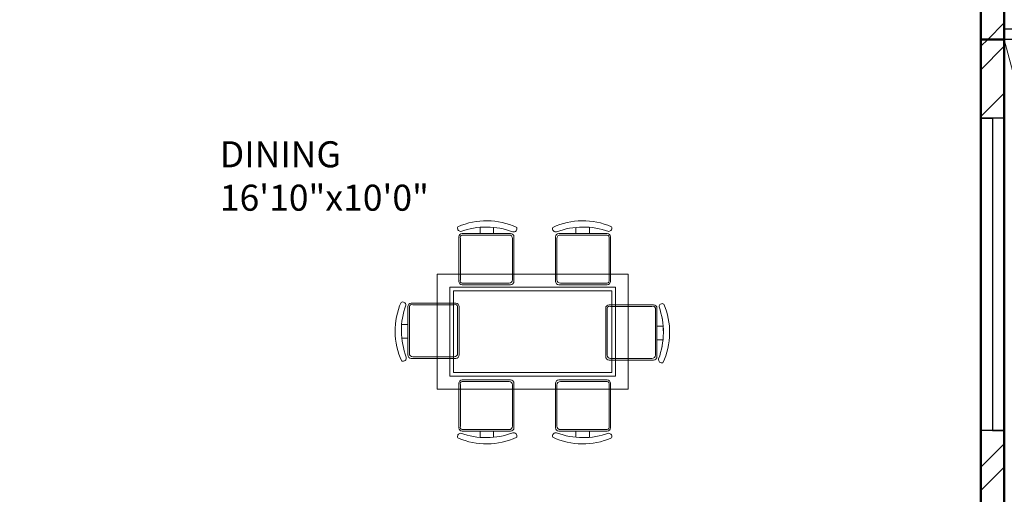
# Model space of a CAD drawing. Units: inches. Extents: x 1901 to 2863, y 888 to 2433.
# Tile 14 of 91: x 2154 to 2343, y 1458 to 1549. Entities that reach past the tile are written whole.
import ezdxf

# ---------------------------------------------------------------- set-up
doc = ezdxf.new("R2010")
doc.units = ezdxf.units.IN
for name, color, linetype, lineweight in [('A-ANNO-SYMB', 8, 'Continuous', 13), ('A-AREA-IDEN', 7, 'Continuous', 18), ('A-FLOR-STRS', 2, 'Continuous', 25), ('A-FURN', 8, 'Continuous', 18), ('A-GLAZ', 3, 'Continuous', 25), ('A-WALL', 7, 'Continuous', 50), ('A-WALL-PATT', 8, 'Continuous', 13)]:
    doc.layers.add(name, color=color, linetype=linetype, lineweight=lineweight)
doc.styles.get("Standard").update_dxf_attribs({"font": 'arial.ttf'})

# ---------------------------------------------------------------- blocks, each defined once
blk = doc.blocks.new('WIN-60')
for p, q in [((0, 4.5), (0, 0)), ((60, 2.25), (60, 4.5)), ((60, 4.5), (60, 0)), ((0, 0), (0, 2.25)), ((0, 2.25), (60, 2.25))]:
    blk.add_line(p, q)

msp = doc.modelspace()

# ---------------------------------------------------------------- hatches: boundary and pattern name
at = {"layer": 'A-WALL-PATT'}
h = msp.add_hatch(dxfattribs=at)
h.set_pattern_fill('ANSI32', color=256)
h.paths.add_polyline_path([(2192.5, 2274.13), (2141.26, 2274.13), (2141.26, 2269.63), (2192.5, 2269.63)])
h.paths.add_polyline_path([(2259.93, 2274.13), (2216.5, 2274.13), (2216.5, 2269.63), (2255.43, 2269.63), (2255.43, 2214.63), (2250.81, 2214.63), (2250.81, 2210.13), (2259.93, 2210.13), (2259.93, 2215.13), (2271.76, 2215.13), (2271.76, 2217.38), (2271.76, 2219.63), (2259.93, 2219.63)])
h.paths.add_polyline_path([(2171.43, 2269.63), (2166.93, 2269.63), (2166.93, 2219.63), (2121.24, 2219.63), (2121.24, 2215.13), (2166.93, 2215.13), (2166.93, 2083.13), (2161.81, 2083.13), (2161.81, 2078.63), (2171.43, 2078.63), (2177, 2078.63), (2177, 2080.88), (2177, 2083.13), (2171.43, 2083.13), (2171.43, 2210.13), (2230.91, 2210.13), (2230.91, 2212.38), (2230.91, 2214.63), (2171.43, 2214.63)])
h.paths.add_polyline_path([(2117.26, 2274.13), (2089.43, 2274.13), (2089.43, 2219.63), (2081.14, 2219.63), (2081.14, 2215.13), (2089.43, 2215.13), (2098, 2215.13), (2098, 2217.38), (2098, 2219.63), (2093.93, 2219.63), (2093.93, 2269.63), (2117.26, 2269.63), (2117.26, 2271.88)])
h.paths.add_polyline_path([(2343.43, 2219.63), (2329.29, 2219.63), (2329.29, 2215.13), (2338.93, 2215.13), (2338.93, 2184.74), (2343.43, 2184.74)])
h.paths.add_polyline_path([(2338.93, 2083.13), (2329.29, 2083.13), (2208.97, 2083.13), (2208.97, 2078.63), (2338.93, 2078.63)])
h.paths.add_polyline_path([(2343.43, 2136.74), (2338.93, 2136.74), (2338.93, 1872.63), (2343.43, 1872.63)])
h.paths.add_polyline_path([(2343.43, 1863.63), (2397.68, 1863.63), (2397.68, 1821.63), (2384.14, 1821.63), (2384.14, 1812.63), (2418.33, 1812.63), (2418.33, 1817.13), (2418.33, 1821.63), (2406.68, 1821.63), (2406.68, 1863.63), (2459.5, 1863.63), (2459.5, 1821.63), (2447.14, 1821.63), (2447.14, 1812.63), (2459.5, 1812.63), (2468.5, 1812.63), (2468.5, 1872.63), (2394.43, 1872.63), (2334.43, 1872.63), (2334.43, 1812.63), (2343.43, 1812.63), (2353.25, 1812.63), (2353.25, 1821.63), (2343.43, 1821.63)])
h.paths.add_polyline_path([(2510.01, 1872.63), (2468.5, 1872.63), (2468.5, 1868.13), (2510.01, 1868.13)])
h.paths.add_polyline_path([(2514.01, 1817.13), (2468.5, 1817.13), (2468.5, 1812.63), (2482.11, 1812.63), (2482.11, 1800.61), (2486.61, 1800.61), (2486.61, 1812.63), (2514.01, 1812.63)])
h.paths.add_polyline_path([(2299.25, 1814.88), (2299.25, 1817.13), (2295.93, 1817.13), (2295.93, 1854.17), (2293.68, 1854.17), (2291.43, 1854.17), (2291.43, 1817.13), (2266.11, 1817.13), (2266.11, 1812.63), (2299.25, 1812.63)])
h.paths.add_polyline_path([(2218.11, 1817.13), (2206.46, 1817.13), (2171.43, 1817.13), (2171.43, 1949.13), (2190.1, 1949.13), (2190.1, 1953.63), (2163.47, 1953.63), (2163.47, 1949.13), (2166.93, 1949.13), (2166.93, 1817.13), (2114.3, 1817.13), (2114.3, 1812.63), (2218.11, 1812.63)])
h.paths.add_polyline_path([(2029.43, 1970.92), (2024.93, 1970.92), (2024.93, 1912.72), (2029.43, 1912.72)])
h.paths.add_polyline_path([(2132.3, 1953.63), (2113.93, 1953.63), (2113.93, 1975.89), (2111.68, 1975.89), (2109.43, 1975.89), (2109.43, 1953.63), (2029.43, 1953.63), (2029.43, 1949.13), (2132.3, 1949.13)])
h.paths.add_polyline_path([(2029.43, 1853.61), (2029.31, 1853.61), (2029.31, 1853.61), (2029.43, 1853.61), (2029.43, 1864.72), (2024.93, 1864.72), (2024.93, 1812.63), (2066.3, 1812.63), (2066.3, 1814.88), (2066.3, 1817.13), (2029.43, 1817.13)])
h.paths.add_polyline_path([(2122.93, 2010.09), (2120.68, 2010.09), (2118.43, 2010.09), (2118.43, 2006.13), (2029.43, 2006.13), (2029.43, 2001.63), (2109.43, 2001.63), (2109.43, 1998.04), (2113.93, 1998.04), (2113.93, 2001.63), (2122.93, 2001.63)])
h.paths.add_polyline_path([(2029.43, 2031.38), (2024.93, 2031.38), (2024.93, 1994.92), (2027.18, 1994.92), (2029.43, 1994.92)])
h.paths.add_polyline_path([(2029.43, 2136.74), (2024.93, 2136.74), (2024.93, 2067.38), (2027.18, 2067.38), (2029.43, 2067.38)])
h.paths.add_polyline_path([(2125.62, 2083.13), (2029.43, 2083.13), (2029.43, 2078.63), (2118.43, 2078.63), (2118.43, 2030.71), (2122.93, 2030.71), (2122.93, 2078.63), (2125.62, 2078.63)])
h.paths.add_polyline_path([(2029.43, 2215.13), (2040.47, 2215.13), (2040.47, 2217.38), (2040.47, 2219.63), (2024.93, 2219.63), (2024.93, 2184.74), (2029.43, 2184.74), (2029.43, 2187.78)])
h.paths.add_polyline_path([(2686.43, 2274.13), (2659.28, 2274.13), (2659.28, 2269.63), (2681.93, 2269.63), (2681.93, 2219.63), (2676.82, 2219.63), (2676.82, 2215.13), (2681.93, 2215.13), (2697.01, 2215.13), (2697.01, 2217.38), (2697.01, 2219.63), (2686.43, 2219.63)])
h.paths.add_polyline_path([(2609.93, 2269.63), (2635.28, 2269.63), (2635.28, 2274.13), (2571.43, 2274.13), (2571.43, 2269.63), (2605.43, 2269.63), (2605.43, 2214.63), (2549.1, 2214.63), (2549.1, 2210.13), (2605.43, 2210.13), (2605.43, 2083.13), (2601.01, 2083.13), (2601.01, 2080.88), (2601.01, 2078.63), (2609.93, 2078.63), (2616.16, 2078.63), (2616.16, 2080.88), (2616.16, 2083.13), (2609.93, 2083.13), (2609.93, 2215.13), (2651.46, 2215.13), (2651.46, 2217.38), (2651.46, 2219.63), (2609.93, 2219.63)])
h.paths.add_polyline_path([(2521.43, 2269.63), (2547.43, 2269.63), (2547.43, 2271.88), (2547.43, 2274.13), (2516.93, 2274.13), (2516.93, 2219.63), (2506.41, 2219.63), (2506.41, 2215.13), (2516.93, 2215.13), (2516.93, 2210.13), (2525.4, 2210.13), (2525.4, 2212.38), (2525.4, 2214.63), (2521.43, 2214.63)])
h.paths.add_polyline_path([(2456.01, 2219.63), (2439.43, 2219.63), (2439.43, 2187.89), (2443.93, 2187.89), (2443.93, 2215.13), (2456.01, 2215.13)])
h.paths.add_polyline_path([(2752.93, 2219.63), (2739.48, 2219.63), (2739.48, 2215.13), (2748.43, 2215.13), (2748.43, 2187.89), (2752.93, 2187.89)])
h.paths.add_polyline_path([(2752.93, 2139.89), (2748.43, 2139.89), (2748.43, 2083.13), (2648.42, 2083.13), (2648.42, 2078.63), (2654.93, 2078.63), (2654.93, 2039.44), (2659.43, 2039.44), (2659.43, 2078.63), (2748.43, 2078.63), (2748.43, 2063.43), (2752.93, 2063.43)])
h.paths.add_polyline_path([(2752.93, 2010.63), (2659.43, 2010.63), (2659.43, 2015.65), (2654.93, 2015.65), (2654.93, 2010.63), (2605.43, 2010.63), (2605.43, 1920.97), (2609.93, 1920.97), (2609.93, 2006.13), (2748.43, 2006.13), (2748.43, 1982.47), (2752.93, 1982.47)])
h.paths.add_polyline_path([(2752.93, 2027.43), (2748.43, 2027.43), (2748.43, 2010.63), (2752.93, 2010.63)])
h.paths.add_polyline_path([(2748.43, 1886.13), (2609.93, 1886.13), (2609.93, 1889.72), (2605.43, 1889.72), (2605.43, 1861.26), (2609.93, 1861.26), (2609.93, 1881.63), (2748.43, 1881.63)])
h.paths.add_polyline_path([(2456.86, 2228.83), (2498.4, 2228.83), (2498.4, 2247.49), (2456.86, 2247.49)], flags=9)
h.paths.add_polyline_path([(2038.6, 2237.42), (2080.17, 2237.42), (2080.17, 2256.08), (2038.6, 2256.08)], flags=9)
h.paths.add_polyline_path([(2292.01, 1062.39), (2539.93, 1062.39), (2539.93, 1099.49), (2292.01, 1099.49)], flags=9)
h.paths.add_polyline_path([(2424.91, 1832.25), (2448.51, 1832.25), (2448.51, 1846.68), (2424.91, 1846.68)], flags=25)
h.paths.add_polyline_path([(2359.08, 1832.25), (2382.68, 1832.25), (2382.68, 1846.68), (2359.08, 1846.68)], flags=25)
h.paths.add_polyline_path([(2352.9, 1684.8), (2367.54, 1684.8), (2367.54, 1697.17), (2352.9, 1697.17)], flags=9)
h.paths.add_polyline_path([(2079.29, 1755.83), (2169.02, 1755.83), (2169.02, 1774.37), (2079.29, 1774.37)], flags=9)
h.paths.add_polyline_path([(2404.09, 1373.86), (2404.09, 1463.59), (2385.54, 1463.59), (2385.54, 1373.86)], flags=9)
h.paths.add_polyline_path([(2268.09, 2236.37), (2309.64, 2236.37), (2309.64, 2255.03), (2268.09, 2255.03)], flags=9)
h.paths.add_polyline_path([(2575.96, 1700.95), (2665.7, 1700.95), (2665.7, 1719.5), (2575.96, 1719.5)], flags=9)
h.paths.add_polyline_path([(2302.96, 1878.47), (2329.52, 1878.47), (2329.52, 1888.78), (2302.96, 1888.78)], flags=9)
h.paths.add_polyline_path([(2097.42, 2240.58), (2126.57, 2240.58), (2126.57, 2259.23), (2097.42, 2259.23)], flags=9)
h.paths.add_polyline_path([(2208.72, 2246.12), (2237.88, 2246.12), (2237.88, 2264.78), (2208.72, 2264.78)], flags=9)
h.paths.add_polyline_path([(2038.15, 1925.96), (2076.99, 1925.96), (2076.99, 1944.62), (2038.15, 1944.62)], flags=9)
h.paths.add_polyline_path([(2239.14, 1926.67), (2288.46, 1926.67), (2288.46, 1945.33), (2239.14, 1945.33)], flags=9)
h.paths.add_polyline_path([(2175.43, 2007.33), (2212.36, 2007.33), (2212.36, 2025.99), (2175.43, 2025.99)], flags=9)
h.paths.add_polyline_path([(2225.03, 2091.79), (2263.87, 2091.79), (2263.87, 2110.45), (2225.03, 2110.45)], flags=9)
h.paths.add_polyline_path([(2035.4, 2098.48), (2074.24, 2098.48), (2074.24, 2117.14), (2035.4, 2117.14)], flags=9)
h.paths.add_polyline_path([(2050.1, 2029.21), (2083.26, 2029.21), (2083.26, 2047.87), (2050.1, 2047.87)], flags=9)
h.paths.add_polyline_path([(2069.68, 1956.72), (2098.83, 1956.72), (2098.83, 1975.38), (2069.68, 1975.38)], flags=25)
h.paths.add_polyline_path([(2328.62, 1753.34), (2361.66, 1753.34), (2361.66, 1771.99), (2328.62, 1771.99)], flags=9)
h.paths.add_polyline_path([(2395.16, 2060.89), (2395.16, 2140.65), (2378.68, 2140.65), (2378.68, 2060.89)], flags=9)
h.paths.add_polyline_path([(2463.73, 2059.02), (2492.89, 2059.02), (2492.89, 2077.68), (2463.73, 2077.68)], flags=9)
h.paths.add_polyline_path([(2458.03, 2181.54), (2496.87, 2181.54), (2496.87, 2200.19), (2458.03, 2200.19)], flags=9)
h.paths.add_polyline_path([(2527.58, 2243.07), (2556.73, 2243.07), (2556.73, 2261.73), (2527.58, 2261.73)], flags=9)
h.paths.add_polyline_path([(2694.46, 2232.77), (2736.03, 2232.77), (2736.03, 2251.42), (2694.46, 2251.42)], flags=9)
h.paths.add_polyline_path([(2637.82, 2249.22), (2666.98, 2249.22), (2666.98, 2267.88), (2637.82, 2267.88)], flags=9)
h.paths.add_polyline_path([(2623.69, 2183.54), (2662.53, 2183.54), (2662.53, 2202.2), (2623.69, 2202.2)], flags=9)
h.paths.add_polyline_path([(2691.97, 2021.5), (2725.12, 2021.5), (2725.12, 2040.16), (2691.97, 2040.16)], flags=9)
h.paths.add_polyline_path([(2621.04, 1975.91), (2662.34, 1975.91), (2662.34, 1994.57), (2621.04, 1994.57)], flags=25)
h.paths.add_polyline_path([(2479.03, 1927.62), (2519.84, 1927.62), (2519.84, 1946.28), (2479.03, 1946.28)], flags=9)
h.paths.add_polyline_path([(2670.94, 1849.08), (2716.01, 1849.08), (2716.01, 1867.73), (2670.94, 1867.73)], flags=9)
h.paths.add_polyline_path([(2523.61, 1782.96), (2550.17, 1782.96), (2550.17, 1793.26), (2523.61, 1793.26)], flags=9)
h.paths.add_polyline_path([(2450.84, 1207.33), (2492.39, 1207.33), (2492.39, 1225.99), (2450.84, 1225.99)], flags=9)
h.paths.add_polyline_path([(2527.75, 1203.84), (2556.91, 1203.84), (2556.91, 1222.5), (2527.75, 1222.5)], flags=9)
h.paths.add_polyline_path([(2639.11, 1207.2), (2668.27, 1207.2), (2668.27, 1225.86), (2639.11, 1225.86)], flags=9)
h.paths.add_polyline_path([(2692.59, 1218.97), (2734.17, 1218.97), (2734.17, 1237.62), (2692.59, 1237.62)], flags=9)
h.paths.add_polyline_path([(2669.27, 1366.33), (2708.11, 1366.33), (2708.11, 1384.99), (2669.27, 1384.99)], flags=9)
h.paths.add_polyline_path([(2463.31, 1358.03), (2502.15, 1358.03), (2502.15, 1376.69), (2463.31, 1376.69)], flags=9)
h.paths.add_polyline_path([(2494.72, 1449.96), (2531.65, 1449.96), (2531.65, 1468.62), (2494.72, 1468.62)], flags=9)
h.paths.add_polyline_path([(2675.57, 1422.16), (2708.72, 1422.16), (2708.72, 1440.81), (2675.57, 1440.81)], flags=9)
h.paths.add_polyline_path([(2685.63, 1493.89), (2714.79, 1493.89), (2714.79, 1512.55), (2685.63, 1512.55)], flags=9)
h.paths.add_polyline_path([(2686.8, 1529.91), (2725.65, 1529.91), (2725.65, 1548.57), (2686.8, 1548.57)], flags=9)
h.paths.add_polyline_path([(2503.65, 1537.99), (2552.97, 1537.99), (2552.97, 1556.65), (2503.65, 1556.65)], flags=9)
h.paths.add_polyline_path([(2291.71, 1643.5), (2318.28, 1643.5), (2318.28, 1653.81), (2291.71, 1653.81)], flags=9)
h.paths.add_polyline_path([(2450.63, 1610.52), (2477.19, 1610.52), (2477.19, 1620.82), (2450.63, 1620.82)], flags=9)
h.paths.add_polyline_path([(2359.99, 1551.81), (2422.25, 1551.81), (2422.25, 1562.12), (2359.99, 1562.12)], flags=9)
h.paths.add_polyline_path([(2280.11, 1249.01), (2321.65, 1249.01), (2321.65, 1267.66), (2280.11, 1267.66)], flags=9)
h.paths.add_polyline_path([(2164.06, 1274.23), (2193.22, 1274.23), (2193.22, 1292.89), (2164.06, 1292.89)], flags=9)
h.paths.add_polyline_path([(2118.21, 1277.69), (2151.25, 1277.69), (2151.25, 1296.35), (2118.21, 1296.35)], flags=9)
h.paths.add_polyline_path([(2031.95, 1268.53), (2073.52, 1268.53), (2073.52, 1287.19), (2031.95, 1287.19)], flags=9)
h.paths.add_polyline_path([(2050.2, 1409.08), (2089.04, 1409.08), (2089.04, 1427.74), (2050.2, 1427.74)], flags=9)
h.paths.add_polyline_path([(2243.74, 1421.03), (2282.58, 1421.03), (2282.58, 1439.69), (2243.74, 1439.69)], flags=9)
h.paths.add_polyline_path([(2190.75, 1509.77), (2231.56, 1509.77), (2231.56, 1528.43), (2190.75, 1528.43)], flags=9)
h.paths.add_polyline_path([(2058.39, 1475.42), (2091.55, 1475.42), (2091.55, 1494.07), (2058.39, 1494.07)], flags=9)
h.paths.add_polyline_path([(2062.45, 1553.09), (2091.6, 1553.09), (2091.6, 1571.75), (2062.45, 1571.75)], flags=9)
h.paths.add_polyline_path([(2219.52, 1590.37), (2266.15, 1590.37), (2266.15, 1609.02), (2219.52, 1609.02)], flags=9)
h.paths.add_polyline_path([(2041.07, 1584.19), (2079.91, 1584.19), (2079.91, 1602.85), (2041.07, 1602.85)], flags=9)
h = msp.add_hatch(dxfattribs=at)
h.set_pattern_fill('ANSI32', color=256)
h.paths.add_polyline_path([(2443.93, 2139.89), (2439.43, 2139.89), (2439.43, 2069.35), (2441.68, 2069.35), (2443.93, 2069.35), (2443.93, 2078.63), (2521.93, 2078.63), (2521.93, 2075.07), (2524.18, 2075.07), (2526.43, 2075.07), (2526.43, 2078.63), (2571.75, 2078.63), (2571.75, 2080.88), (2571.75, 2083.13), (2443.93, 2083.13)])
h.paths.add_polyline_path([(2526.43, 2054.63), (2524.18, 2054.63), (2521.93, 2054.63), (2521.93, 2030.63), (2443.93, 2030.63), (2443.93, 2045.35), (2439.43, 2045.35), (2439.43, 1983.87), (2443.93, 1983.87), (2443.93, 2026.13), (2521.93, 2026.13), (2526.43, 2026.13)])
h.paths.add_polyline_path([(2443.93, 1923.87), (2439.43, 1923.87), (2439.43, 1872.63), (2443.93, 1872.63)])
h.paths.add_polyline_path([(2636.23, 1766.13), (2609.93, 1766.13), (2609.93, 1779.79), (2605.43, 1779.79), (2605.43, 1766.13), (2486.61, 1766.13), (2486.61, 1770.67), (2482.11, 1770.67), (2482.11, 1766.13), (2482.11, 1761.63), (2636.23, 1761.63), (2636.23, 1763.88)])
h.paths.add_polyline_path([(2519.54, 1663.38), (2519.54, 1665.63), (2494.93, 1665.63), (2481.83, 1665.63), (2481.83, 1663.38), (2481.83, 1661.13), (2490.43, 1661.13), (2490.43, 1640.16), (2494.93, 1640.16), (2494.93, 1661.13), (2519.54, 1661.13)])
h.paths.add_polyline_path([(2443.93, 1712.13), (2443.93, 1716.63), (2414.46, 1716.63), (2414.46, 1712.13), (2439.43, 1712.13), (2439.43, 1545.51), (2443.93, 1545.51), (2443.93, 1661.13), (2448.47, 1661.13), (2448.47, 1665.63), (2443.93, 1665.63)])
h.paths.add_polyline_path([(2343.43, 1712.13), (2365.52, 1712.13), (2365.52, 1714.38), (2365.52, 1716.63), (2333.87, 1716.63), (2333.87, 1714.38), (2333.87, 1712.13), (2338.93, 1712.13), (2338.93, 1575.63), (2338.93, 1545.51), (2343.43, 1545.51), (2343.43, 1547.51), (2343.43, 1580.13)])
h.paths.add_polyline_path([(2752.93, 1665.63), (2579.54, 1665.63), (2579.54, 1661.13), (2615.93, 1661.13), (2615.93, 1529.13), (2598.93, 1529.13), (2598.93, 1524.63), (2623.13, 1524.63), (2623.13, 1526.88), (2623.13, 1529.13), (2620.43, 1529.13), (2620.43, 1661.13), (2748.43, 1661.13), (2748.43, 1633.5), (2752.93, 1633.5)])
h.paths.add_polyline_path([(2752.93, 1419.93), (2748.43, 1419.93), (2748.43, 1400.13), (2659.43, 1400.13), (2659.43, 1444.33), (2657.18, 1444.33), (2654.93, 1444.33), (2654.93, 1400.13), (2643.65, 1400.13), (2643.65, 1395.63), (2748.43, 1395.63), (2748.43, 1364.04), (2752.93, 1364.04)])
h.paths.add_polyline_path([(2752.93, 1492.88), (2748.43, 1492.88), (2748.43, 1476.63), (2667.43, 1476.63), (2667.43, 1479.71), (2665.18, 1479.71), (2662.93, 1479.71), (2662.93, 1476.63), (2654.93, 1476.63), (2654.93, 1469.54), (2659.43, 1469.54), (2659.43, 1472.13), (2748.43, 1472.13), (2748.43, 1455.93), (2752.93, 1455.93)])
h.paths.add_polyline_path([(2752.93, 1304.04), (2748.43, 1304.04), (2748.43, 1263.63), (2738.66, 1263.63), (2738.66, 1259.13), (2752.93, 1259.13)])
h.paths.add_polyline_path([(2685.93, 1259.13), (2695.49, 1259.13), (2695.49, 1261.38), (2695.49, 1263.63), (2677.84, 1263.63), (2677.84, 1261.38), (2677.84, 1259.13), (2681.43, 1259.13), (2681.43, 1203.63), (2653.28, 1203.63), (2653.28, 1199.13), (2685.93, 1199.13), (2685.93, 1203.63)])
h.paths.add_polyline_path([(2609.43, 1395.63), (2611.85, 1395.63), (2611.85, 1400.13), (2598.89, 1400.13), (2598.89, 1397.88), (2598.89, 1395.63), (2604.93, 1395.63), (2604.93, 1268.13), (2554.73, 1268.13), (2554.73, 1265.88), (2554.73, 1263.63), (2604.93, 1263.63), (2604.93, 1203.63), (2571.31, 1203.63), (2571.31, 1199.13), (2604.93, 1199.13), (2629.28, 1199.13), (2629.28, 1201.38), (2629.28, 1203.63), (2609.43, 1203.63), (2609.43, 1258.63), (2609.43, 1259.13), (2654.8, 1259.13), (2654.8, 1263.63), (2609.43, 1263.63)])
h.paths.add_polyline_path([(2443.93, 1304.04), (2439.43, 1304.04), (2439.43, 1259.13), (2443.93, 1259.13), (2456.16, 1259.13), (2456.16, 1261.38), (2456.16, 1263.63), (2443.93, 1263.63)])
h.paths.add_polyline_path([(2525.43, 1263.63), (2531.78, 1263.63), (2531.78, 1268.13), (2520.93, 1268.13), (2520.93, 1263.63), (2511.41, 1263.63), (2511.41, 1259.13), (2520.93, 1259.13), (2520.93, 1199.13), (2547.31, 1199.13), (2547.31, 1201.38), (2547.31, 1203.63), (2525.43, 1203.63)])
h.paths.add_polyline_path([(2443.93, 1434.84), (2439.43, 1434.84), (2439.43, 1364.04), (2441.68, 1364.04), (2443.93, 1364.04)])
h.paths.add_polyline_path([(2567.13, 1400.13), (2443.93, 1400.13), (2443.93, 1395.63), (2567.13, 1395.63)])
h.paths.add_polyline_path([(2443.93, 1545.51), (2439.43, 1545.51), (2439.43, 1494.84), (2443.93, 1494.84)])
h.paths.add_polyline_path([(2494.93, 1553.35), (2492.68, 1553.35), (2490.43, 1553.35), (2490.43, 1524.63), (2494.93, 1524.63), (2525.94, 1524.63), (2525.94, 1526.88), (2525.94, 1529.13), (2494.93, 1529.13)])
h.paths.add_polyline_path([(2752.93, 1573.5), (2748.43, 1573.5), (2748.43, 1529.13), (2657.76, 1529.13), (2657.76, 1524.63), (2662.93, 1524.63), (2662.93, 1498.63), (2667.43, 1498.63), (2667.43, 1524.63), (2748.43, 1524.63), (2748.43, 1516.88), (2752.93, 1516.88)])
h.paths.add_polyline_path([(2038.6, 2237.42), (2080.17, 2237.42), (2080.17, 2256.08), (2038.6, 2256.08)], flags=9)
h.paths.add_polyline_path([(2292.01, 1062.39), (2539.93, 1062.39), (2539.93, 1099.49), (2292.01, 1099.49)], flags=9)
h.paths.add_polyline_path([(2424.91, 1832.25), (2448.51, 1832.25), (2448.51, 1846.68), (2424.91, 1846.68)], flags=9)
h.paths.add_polyline_path([(2359.08, 1832.25), (2382.68, 1832.25), (2382.68, 1846.68), (2359.08, 1846.68)], flags=9)
h.paths.add_polyline_path([(2352.9, 1684.8), (2367.54, 1684.8), (2367.54, 1697.17), (2352.9, 1697.17)], flags=9)
h.paths.add_polyline_path([(2079.29, 1755.83), (2169.02, 1755.83), (2169.02, 1774.37), (2079.29, 1774.37)], flags=9)
h.paths.add_polyline_path([(2404.09, 1373.86), (2404.09, 1463.59), (2385.54, 1463.59), (2385.54, 1373.86)], flags=9)
h.paths.add_polyline_path([(2268.09, 2236.37), (2309.64, 2236.37), (2309.64, 2255.03), (2268.09, 2255.03)], flags=9)
h.paths.add_polyline_path([(2575.96, 1700.95), (2665.7, 1700.95), (2665.7, 1719.5), (2575.96, 1719.5)], flags=9)
h.paths.add_polyline_path([(2302.96, 1878.47), (2329.52, 1878.47), (2329.52, 1888.78), (2302.96, 1888.78)], flags=9)
h.paths.add_polyline_path([(2097.42, 2240.58), (2126.57, 2240.58), (2126.57, 2259.23), (2097.42, 2259.23)], flags=9)
h.paths.add_polyline_path([(2208.72, 2246.12), (2237.88, 2246.12), (2237.88, 2264.78), (2208.72, 2264.78)], flags=9)
h.paths.add_polyline_path([(2038.15, 1925.96), (2076.99, 1925.96), (2076.99, 1944.62), (2038.15, 1944.62)], flags=9)
h.paths.add_polyline_path([(2239.14, 1926.67), (2288.46, 1926.67), (2288.46, 1945.33), (2239.14, 1945.33)], flags=9)
h.paths.add_polyline_path([(2175.43, 2007.33), (2212.36, 2007.33), (2212.36, 2025.99), (2175.43, 2025.99)], flags=9)
h.paths.add_polyline_path([(2225.03, 2091.79), (2263.87, 2091.79), (2263.87, 2110.45), (2225.03, 2110.45)], flags=9)
h.paths.add_polyline_path([(2035.4, 2098.48), (2074.24, 2098.48), (2074.24, 2117.14), (2035.4, 2117.14)], flags=9)
h.paths.add_polyline_path([(2050.1, 2029.21), (2083.26, 2029.21), (2083.26, 2047.87), (2050.1, 2047.87)], flags=9)
h.paths.add_polyline_path([(2069.68, 1956.72), (2098.83, 1956.72), (2098.83, 1975.38), (2069.68, 1975.38)], flags=9)
h.paths.add_polyline_path([(2328.62, 1753.34), (2361.66, 1753.34), (2361.66, 1771.99), (2328.62, 1771.99)], flags=9)
h.paths.add_polyline_path([(2395.16, 2060.89), (2395.16, 2140.65), (2378.68, 2140.65), (2378.68, 2060.89)], flags=9)
h.paths.add_polyline_path([(2463.73, 2059.02), (2492.89, 2059.02), (2492.89, 2077.68), (2463.73, 2077.68)], flags=9)
h.paths.add_polyline_path([(2458.03, 2181.54), (2496.87, 2181.54), (2496.87, 2200.19), (2458.03, 2200.19)], flags=9)
h.paths.add_polyline_path([(2456.86, 2228.83), (2498.4, 2228.83), (2498.4, 2247.49), (2456.86, 2247.49)], flags=9)
h.paths.add_polyline_path([(2527.58, 2243.07), (2556.73, 2243.07), (2556.73, 2261.73), (2527.58, 2261.73)], flags=9)
h.paths.add_polyline_path([(2694.46, 2232.77), (2736.03, 2232.77), (2736.03, 2251.42), (2694.46, 2251.42)], flags=9)
h.paths.add_polyline_path([(2637.82, 2249.22), (2666.98, 2249.22), (2666.98, 2267.88), (2637.82, 2267.88)], flags=9)
h.paths.add_polyline_path([(2623.69, 2183.54), (2662.53, 2183.54), (2662.53, 2202.2), (2623.69, 2202.2)], flags=9)
h.paths.add_polyline_path([(2691.97, 2021.5), (2725.12, 2021.5), (2725.12, 2040.16), (2691.97, 2040.16)], flags=9)
h.paths.add_polyline_path([(2621.04, 1975.91), (2662.34, 1975.91), (2662.34, 1994.57), (2621.04, 1994.57)], flags=9)
h.paths.add_polyline_path([(2479.03, 1927.62), (2519.84, 1927.62), (2519.84, 1946.28), (2479.03, 1946.28)], flags=9)
h.paths.add_polyline_path([(2670.94, 1849.08), (2716.01, 1849.08), (2716.01, 1867.73), (2670.94, 1867.73)], flags=9)
h.paths.add_polyline_path([(2523.61, 1782.96), (2550.17, 1782.96), (2550.17, 1793.26), (2523.61, 1793.26)], flags=9)
h.paths.add_polyline_path([(2450.84, 1207.33), (2492.39, 1207.33), (2492.39, 1225.99), (2450.84, 1225.99)], flags=9)
h.paths.add_polyline_path([(2527.75, 1203.84), (2556.91, 1203.84), (2556.91, 1222.5), (2527.75, 1222.5)], flags=9)
h.paths.add_polyline_path([(2639.11, 1207.2), (2668.27, 1207.2), (2668.27, 1225.86), (2639.11, 1225.86)], flags=9)
h.paths.add_polyline_path([(2692.59, 1218.97), (2734.17, 1218.97), (2734.17, 1237.62), (2692.59, 1237.62)], flags=9)
h.paths.add_polyline_path([(2669.27, 1366.33), (2708.11, 1366.33), (2708.11, 1384.99), (2669.27, 1384.99)], flags=25)
h.paths.add_polyline_path([(2463.31, 1358.03), (2502.15, 1358.03), (2502.15, 1376.69), (2463.31, 1376.69)], flags=9)
h.paths.add_polyline_path([(2494.72, 1449.96), (2531.65, 1449.96), (2531.65, 1468.62), (2494.72, 1468.62)], flags=9)
h.paths.add_polyline_path([(2675.57, 1422.16), (2708.72, 1422.16), (2708.72, 1440.81), (2675.57, 1440.81)], flags=25)
h.paths.add_polyline_path([(2685.63, 1493.89), (2714.79, 1493.89), (2714.79, 1512.55), (2685.63, 1512.55)], flags=9)
h.paths.add_polyline_path([(2686.8, 1529.91), (2725.65, 1529.91), (2725.65, 1548.57), (2686.8, 1548.57)], flags=25)
h.paths.add_polyline_path([(2503.65, 1537.99), (2552.97, 1537.99), (2552.97, 1556.65), (2503.65, 1556.65)], flags=9)
h.paths.add_polyline_path([(2291.71, 1643.5), (2318.28, 1643.5), (2318.28, 1653.81), (2291.71, 1653.81)], flags=9)
h.paths.add_polyline_path([(2450.63, 1610.52), (2477.19, 1610.52), (2477.19, 1620.82), (2450.63, 1620.82)], flags=9)
h.paths.add_polyline_path([(2359.99, 1551.81), (2422.25, 1551.81), (2422.25, 1562.12), (2359.99, 1562.12)], flags=9)
h.paths.add_polyline_path([(2280.11, 1249.01), (2321.65, 1249.01), (2321.65, 1267.66), (2280.11, 1267.66)], flags=9)
h.paths.add_polyline_path([(2164.06, 1274.23), (2193.22, 1274.23), (2193.22, 1292.89), (2164.06, 1292.89)], flags=9)
h.paths.add_polyline_path([(2118.21, 1277.69), (2151.25, 1277.69), (2151.25, 1296.35), (2118.21, 1296.35)], flags=9)
h.paths.add_polyline_path([(2031.95, 1268.53), (2073.52, 1268.53), (2073.52, 1287.19), (2031.95, 1287.19)], flags=9)
h.paths.add_polyline_path([(2050.2, 1409.08), (2089.04, 1409.08), (2089.04, 1427.74), (2050.2, 1427.74)], flags=9)
h.paths.add_polyline_path([(2243.74, 1421.03), (2282.58, 1421.03), (2282.58, 1439.69), (2243.74, 1439.69)], flags=9)
h.paths.add_polyline_path([(2190.75, 1509.77), (2231.56, 1509.77), (2231.56, 1528.43), (2190.75, 1528.43)], flags=9)
h.paths.add_polyline_path([(2058.39, 1475.42), (2091.55, 1475.42), (2091.55, 1494.07), (2058.39, 1494.07)], flags=9)
h.paths.add_polyline_path([(2062.45, 1553.09), (2091.6, 1553.09), (2091.6, 1571.75), (2062.45, 1571.75)], flags=9)
h.paths.add_polyline_path([(2219.52, 1590.37), (2266.15, 1590.37), (2266.15, 1609.02), (2219.52, 1609.02)], flags=9)
h.paths.add_polyline_path([(2041.07, 1584.19), (2079.91, 1584.19), (2079.91, 1602.85), (2041.07, 1602.85)], flags=9)
h = msp.add_hatch(dxfattribs=at)
h.set_pattern_fill('ANSI32', color=256)
h.paths.add_polyline_path([(2182.93, 1716.63), (2024.93, 1716.63), (2024.93, 1681.7), (2029.33, 1681.7), (2029.33, 1712.13), (2154.33, 1712.13), (2154.33, 1580.13), (2148.52, 1580.13), (2148.52, 1577.88), (2148.52, 1575.63), (2194.93, 1575.63), (2194.93, 1580.13), (2158.83, 1580.13), (2158.83, 1712.13), (2182.93, 1712.13)])
h.paths.add_polyline_path([(2301.07, 1716.63), (2242.93, 1716.63), (2242.93, 1712.13), (2283.83, 1712.13), (2283.83, 1685.54), (2288.33, 1685.54), (2288.33, 1712.13), (2301.07, 1712.13)])
h.paths.add_polyline_path([(2288.33, 1600.41), (2286.08, 1600.41), (2283.83, 1600.41), (2283.83, 1580.13), (2270.6, 1580.13), (2270.6, 1575.63), (2288.33, 1575.63)])
h.paths.add_polyline_path([(2295.93, 1953.63), (2271.45, 1953.63), (2271.45, 1949.13), (2291.43, 1949.13), (2291.43, 1941.24), (2295.93, 1941.24)])
h.paths.add_polyline_path([(2098.38, 1244.13), (2082.33, 1244.13), (2082.33, 1302.13), (2086.52, 1302.13), (2086.52, 1306.63), (2067.46, 1306.63), (2067.46, 1302.13), (2077.83, 1302.13), (2077.83, 1239.63), (2098.38, 1239.63), (2098.38, 1241.88)])
h.paths.add_polyline_path([(2217.31, 1306.63), (2158.83, 1306.63), (2158.83, 1451.63), (2162.72, 1451.63), (2162.72, 1453.88), (2162.72, 1456.13), (2154.33, 1456.13), (2154.33, 1443.13), (2151.91, 1443.13), (2151.91, 1438.63), (2154.33, 1438.63), (2154.33, 1306.63), (2109.31, 1306.63), (2109.31, 1304.38), (2109.31, 1302.13), (2154.33, 1302.13), (2154.33, 1244.13), (2122.38, 1244.13), (2122.38, 1239.63), (2154.33, 1239.63), (2154.33, 1223.63), (2163.33, 1223.63), (2181.01, 1223.63), (2181.01, 1225.88), (2181.01, 1228.13), (2163.33, 1228.13), (2163.33, 1258.22), (2158.83, 1258.22), (2158.83, 1302.13), (2217.31, 1302.13)])
h.paths.add_polyline_path([(2259.99, 1306.63), (2238.3, 1306.63), (2238.3, 1304.38), (2238.3, 1302.13), (2242.83, 1302.13), (2242.83, 1228.13), (2205.01, 1228.13), (2205.01, 1223.63), (2247.33, 1223.63), (2247.33, 1302.13), (2259.99, 1302.13), (2259.99, 1304.38)])
h.paths.add_polyline_path([(2343.43, 1361.7), (2338.93, 1361.7), (2338.93, 1306.63), (2322.38, 1306.63), (2322.38, 1302.13), (2343.43, 1302.13)])
h.paths.add_polyline_path([(2343.43, 1470.4), (2338.93, 1470.4), (2338.93, 1456.13), (2193.73, 1456.13), (2193.73, 1453.88), (2193.73, 1451.63), (2338.93, 1451.63), (2338.93, 1421.7), (2343.43, 1421.7)])
h.paths.add_polyline_path([(2343.43, 1545.51), (2338.93, 1545.51), (2338.93, 1530.4), (2343.43, 1530.4)])
h.paths.add_polyline_path([(2029.33, 1466.83), (2024.93, 1466.83), (2024.93, 1409.82), (2029.33, 1409.82)])
h.paths.add_polyline_path([(2122.84, 1440.88), (2122.84, 1443.13), (2121.83, 1443.13), (2121.83, 1498.18), (2119.58, 1498.18), (2117.33, 1498.18), (2117.33, 1443.13), (2029.33, 1443.13), (2029.33, 1438.63), (2122.84, 1438.63)])
h.paths.add_polyline_path([(2029.33, 1543.05), (2024.93, 1543.05), (2024.93, 1502.83), (2029.33, 1502.83)])
h.paths.add_polyline_path([(2029.33, 1621.7), (2024.93, 1621.7), (2024.93, 1567.05), (2027.13, 1567.05), (2029.33, 1567.05), (2029.33, 1575.63), (2109.33, 1575.63), (2109.33, 1554.71), (2113.83, 1554.71), (2113.83, 1575.63), (2115.8, 1575.63), (2115.8, 1577.88), (2115.8, 1580.13), (2029.33, 1580.13)])
h.paths.add_polyline_path([(2121.83, 1527.63), (2117.33, 1527.63), (2113.83, 1527.63), (2113.83, 1533.01), (2111.58, 1533.01), (2109.33, 1533.01), (2109.33, 1527.63), (2029.33, 1527.63), (2029.33, 1523.13), (2117.33, 1523.13), (2117.33, 1519.43), (2121.83, 1519.43)])
h.paths.add_polyline_path([(2029.33, 1349.82), (2024.93, 1349.82), (2024.93, 1302.13), (2036.28, 1302.13), (2036.28, 1306.63), (2029.33, 1306.63)])

# ---------------------------------------------------------------- linework, layer by layer
at = {"layer": 'A-ANNO-SYMB'}
msp.add_line((2343.43, 1545.51), (2439.43, 1181.13), dxfattribs=at)
at = {"layer": 'A-FLOR-STRS'}
for p, q in [((2343.43, 1545.51), (2343.43, 1547.51)), ((2343.43, 1547.51), (2439.43, 1547.51)), ((2439.43, 1545.51), (2343.43, 1545.51))]:
    msp.add_line(p, q, dxfattribs=at)
at = {"layer": 'A-FURN'}
for points in [[(2239.02, 1508.63, -0.175809), (2249.03, 1508.55, 0.578392), (2249.78, 1509.39, 0.214524), (2238.49, 1509.54, 0.552014), (2239.02, 1508.63, -0.065079)], [(2239.02, 1508.63, -0.175809), (2249.03, 1508.55, 0.578392), (2249.78, 1509.39, 0.214524), (2238.49, 1509.54, 0.552014), (2239.02, 1508.63, -0.065079)], [(2245.34, 1508.23), (2245.34, 1509.4, -0.064759)], [(2245.34, 1508.23), (2245.34, 1509.4, -0.064759)], [(2257.45, 1508.55, -0.578392), (2256.69, 1509.39, -0.214524), (2267.98, 1509.54, -0.552014), (2267.45, 1508.63, 0.175809), (2257.45, 1508.55)], [(2257.45, 1508.55, -0.578392), (2256.69, 1509.39, -0.214524), (2267.98, 1509.54, -0.552014), (2267.45, 1508.63, 0.175809), (2257.45, 1508.55)], [(2261.13, 1508.23), (2261.13, 1509.4, 0.064759)], [(2261.13, 1508.23), (2261.13, 1509.4, 0.064759)], [(2248.6, 1508.23), (2239.31, 1508.23, 0.414214), (2238.66, 1507.58), (2238.66, 1499.04, 0.414214), (2239.31, 1498.39), (2248.6, 1498.39, 0.414214), (2249.25, 1499.04), (2249.25, 1507.58, 0.414214), (2248.6, 1508.23)], [(2248.6, 1508.23), (2239.31, 1508.23, 0.414214), (2238.66, 1507.58), (2238.66, 1499.04, 0.414214), (2239.31, 1498.39), (2248.6, 1498.39, 0.414214), (2249.25, 1499.04), (2249.25, 1507.58, 0.414214), (2248.6, 1508.23)], [(2267.16, 1508.23, -0.414214), (2267.81, 1507.58), (2267.81, 1499.04, -0.414214), (2267.16, 1498.39), (2257.87, 1498.39, -0.414214), (2257.22, 1499.04), (2257.22, 1507.58, -0.414214), (2257.87, 1508.23), (2267.16, 1508.23)], [(2267.16, 1508.23, -0.414214), (2267.81, 1507.58), (2267.81, 1499.04, -0.414214), (2267.16, 1498.39), (2257.87, 1498.39, -0.414214), (2257.22, 1499.04), (2257.22, 1507.58, -0.414214), (2257.87, 1508.23), (2267.16, 1508.23)], [(2228.56, 1484.47, -0.578392), (2227.72, 1483.72, -0.214524), (2227.57, 1495.01, -0.552014), (2228.48, 1494.48, 0.175809), (2228.56, 1484.47)], [(2228.56, 1484.47, -0.578392), (2227.72, 1483.72, -0.214524), (2227.57, 1495.01, -0.552014), (2228.48, 1494.48, 0.175809), (2228.56, 1484.47)], [(2228.88, 1494.18, -0.414214), (2229.53, 1494.83), (2238.07, 1494.83, -0.414214), (2238.72, 1494.18), (2238.72, 1484.9, -0.414214), (2238.07, 1484.25), (2229.53, 1484.25, -0.414214), (2228.88, 1484.9), (2228.88, 1494.18)], [(2228.88, 1494.18, -0.414214), (2229.53, 1494.83), (2238.07, 1494.83, -0.414214), (2238.72, 1494.18), (2238.72, 1484.9, -0.414214), (2238.07, 1484.25), (2229.53, 1484.25, -0.414214), (2228.88, 1484.9), (2228.88, 1494.18)], [(2276.71, 1493.87, 0.414214), (2276.06, 1494.52), (2267.52, 1494.52, 0.414214), (2266.87, 1493.87), (2266.87, 1484.58, 0.414214), (2267.52, 1483.93), (2276.06, 1483.93, 0.414214), (2276.71, 1484.58), (2276.71, 1493.87)], [(2276.71, 1493.87, 0.414214), (2276.06, 1494.52), (2267.52, 1494.52, 0.414214), (2266.87, 1493.87), (2266.87, 1484.58, 0.414214), (2267.52, 1483.93), (2276.06, 1483.93, 0.414214), (2276.71, 1484.58), (2276.71, 1493.87)], [(2277.11, 1494.16, -0.175809), (2277.03, 1484.16, 0.578392), (2277.86, 1483.4, 0.214524), (2278.02, 1494.69, 0.552014), (2277.11, 1494.16, -0.065079)], [(2277.11, 1494.16, -0.175809), (2277.03, 1484.15, 0.578392), (2277.86, 1483.4, 0.214524), (2278.02, 1494.69, 0.552014), (2277.11, 1494.16, -0.065079)], [(2228.88, 1488.16), (2227.71, 1488.16, 0.064759)], [(2228.88, 1488.16), (2227.71, 1488.16, 0.064759)], [(2276.71, 1487.84), (2277.88, 1487.84, -0.064759)], [(2276.71, 1487.84), (2277.88, 1487.84, -0.064759)], [(2248.6, 1470.27), (2239.31, 1470.27, -0.414214), (2238.66, 1470.92), (2238.66, 1479.46, -0.414214), (2239.31, 1480.11), (2248.6, 1480.11, -0.414214), (2249.25, 1479.46), (2249.25, 1470.92, -0.414214), (2248.6, 1470.27)], [(2248.6, 1470.27), (2239.31, 1470.27, -0.414214), (2238.66, 1470.92), (2238.66, 1479.46, -0.414214), (2239.31, 1480.11), (2248.6, 1480.11, -0.414214), (2249.25, 1479.46), (2249.25, 1470.92, -0.414214), (2248.6, 1470.27)], [(2267.16, 1470.27, 0.414214), (2267.81, 1470.92), (2267.81, 1479.46, 0.414214), (2267.16, 1480.11), (2257.87, 1480.11, 0.414214), (2257.22, 1479.46), (2257.22, 1470.92, 0.414214), (2257.87, 1470.27), (2267.16, 1470.27)], [(2267.16, 1470.27, 0.414214), (2267.81, 1470.92), (2267.81, 1479.46, 0.414214), (2267.16, 1480.11), (2257.87, 1480.11, 0.414214), (2257.22, 1479.46), (2257.22, 1470.92, 0.414214), (2257.87, 1470.27), (2267.16, 1470.27)], [(2249.03, 1469.94, -0.578392), (2249.78, 1469.11, -0.214524), (2238.49, 1468.96, -0.552014), (2239.02, 1469.87, 0.175809), (2249.03, 1469.94)], [(2249.03, 1469.94, -0.578392), (2249.78, 1469.11, -0.214524), (2238.49, 1468.96, -0.552014), (2239.02, 1469.87, 0.175809), (2249.03, 1469.94)], [(2245.34, 1470.27), (2245.34, 1469.1, 0.064759)], [(2245.34, 1470.27), (2245.34, 1469.1, 0.064759)], [(2267.45, 1469.87, -0.175809), (2257.45, 1469.94, 0.578392), (2256.69, 1469.11, 0.214524), (2267.98, 1468.96, 0.552014), (2267.45, 1469.87, -0.065079)], [(2267.45, 1469.87, -0.175809), (2257.45, 1469.94, 0.578392), (2256.69, 1469.11, 0.214524), (2267.98, 1468.96, 0.552014), (2267.45, 1469.87, -0.065079)], [(2261.13, 1470.27), (2261.13, 1469.1, -0.064759)], [(2261.13, 1470.27), (2261.13, 1469.1, -0.064759)]]:
    msp.add_lwpolyline(points, format="xyb", dxfattribs=at)
for points in [[(2242.74, 1509.42), (2242.74, 1508.23)], [(2242.74, 1509.42), (2242.74, 1508.23)], [(2263.73, 1509.42), (2263.73, 1508.23)], [(2263.73, 1509.42), (2263.73, 1508.23)], [(2227.69, 1490.76), (2228.88, 1490.76)], [(2227.69, 1490.76), (2228.88, 1490.76)], [(2277.9, 1490.44), (2276.71, 1490.44)], [(2277.9, 1490.44), (2276.71, 1490.44)], [(2242.74, 1469.07), (2242.74, 1470.27)], [(2242.74, 1469.07), (2242.74, 1470.27)], [(2263.73, 1469.07), (2263.73, 1470.27)], [(2263.73, 1469.07), (2263.73, 1470.27)]]:
    msp.add_lwpolyline(points, dxfattribs=at)
for points in [[(2239.32, 1507.94), (2248.31, 1507.94, -0.414214), (2248.96, 1507.29), (2248.96, 1499.33, -0.414214), (2248.31, 1498.68), (2239.32, 1498.68, -0.512069), (2238.96, 1499.33), (2238.96, 1507.29, -0.512069)], [(2239.32, 1507.94), (2248.31, 1507.94, -0.414214), (2248.96, 1507.29), (2248.96, 1499.33, -0.414214), (2248.31, 1498.68), (2239.32, 1498.68, -0.512069), (2238.96, 1499.33), (2238.96, 1507.29, -0.512069)], [(2267.15, 1507.94), (2258.16, 1507.94, 0.414214), (2257.51, 1507.29), (2257.51, 1499.33, 0.414214), (2258.16, 1498.68), (2267.15, 1498.68, 0.512069), (2267.52, 1499.33), (2267.52, 1507.29, 0.512069)], [(2267.15, 1507.94), (2258.16, 1507.94, 0.414214), (2257.51, 1507.29), (2257.51, 1499.33, 0.414214), (2258.16, 1498.68), (2267.15, 1498.68, 0.512069), (2267.52, 1499.33), (2267.52, 1507.29, 0.512069)], [(2229.17, 1494.18), (2229.17, 1485.19, 0.414214), (2229.82, 1484.54), (2237.78, 1484.54, 0.414214), (2238.43, 1485.19), (2238.43, 1494.18, 0.512069), (2237.78, 1494.54), (2229.82, 1494.54, 0.512069)], [(2229.17, 1494.18), (2229.17, 1485.19, 0.414214), (2229.82, 1484.54), (2237.78, 1484.54, 0.414214), (2238.43, 1485.19), (2238.43, 1494.18, 0.512069), (2237.78, 1494.54), (2229.82, 1494.54, 0.512069)], [(2276.41, 1493.86), (2276.41, 1484.87, -0.414214), (2275.76, 1484.22), (2267.81, 1484.22, -0.414214), (2267.16, 1484.87), (2267.16, 1493.86, -0.512069), (2267.81, 1494.22), (2275.76, 1494.22, -0.512069)], [(2276.41, 1493.86), (2276.41, 1484.87, -0.414214), (2275.76, 1484.22), (2267.81, 1484.22, -0.414214), (2267.16, 1484.87), (2267.16, 1493.86, -0.512069), (2267.81, 1494.22), (2275.76, 1494.22, -0.512069)], [(2239.32, 1470.56), (2248.31, 1470.56, 0.414214), (2248.96, 1471.21), (2248.96, 1479.17, 0.414214), (2248.31, 1479.82), (2239.32, 1479.82, 0.512069), (2238.96, 1479.17), (2238.96, 1471.21, 0.512069)], [(2239.32, 1470.56), (2248.31, 1470.56, 0.414214), (2248.96, 1471.21), (2248.96, 1479.17, 0.414214), (2248.31, 1479.82), (2239.32, 1479.82, 0.512069), (2238.96, 1479.17), (2238.96, 1471.21, 0.512069)], [(2267.15, 1470.56), (2258.16, 1470.56, -0.414214), (2257.51, 1471.21), (2257.51, 1479.17, -0.414214), (2258.16, 1479.82), (2267.15, 1479.82, -0.512069), (2267.52, 1479.17), (2267.52, 1471.21, -0.512069)], [(2267.15, 1470.56), (2258.16, 1470.56, -0.414214), (2257.51, 1471.21), (2257.51, 1479.17, -0.414214), (2258.16, 1479.82), (2267.15, 1479.82, -0.512069), (2267.52, 1479.17), (2267.52, 1471.21, -0.512069)]]:
    msp.add_lwpolyline(points, format="xyb", close=True, dxfattribs=at)
for points in [[(2234.48, 1500.39), (2271.21, 1500.39), (2271.21, 1478.35), (2234.48, 1478.35)], [(2234.48, 1500.39), (2271.21, 1500.39), (2271.21, 1478.35), (2234.48, 1478.35)], [(2236.93, 1497.94), (2268.76, 1497.94), (2268.76, 1480.8), (2236.93, 1480.8)], [(2236.93, 1497.94), (2268.76, 1497.94), (2268.76, 1480.8), (2236.93, 1480.8)], [(2237.66, 1497.2), (2268.02, 1497.2), (2268.02, 1481.53), (2237.66, 1481.53)], [(2237.66, 1497.2), (2268.02, 1497.2), (2268.02, 1481.53), (2237.66, 1481.53)]]:
    msp.add_lwpolyline(points, close=True, dxfattribs=at)
at = {"layer": 'A-WALL'}
for p, q in [((2343.43, 1302.13), (2343.43, 1580.13)), ((2338.93, 1575.63), (2338.93, 1456.13)), ((2338.93, 1545.51), (2343.43, 1545.51))]:
    msp.add_line(p, q, dxfattribs=at)

# ---------------------------------------------------------------- block references
at = {"layer": 'A-GLAZ', "rotation": 270.0000000000013}
msp.add_blockref('WIN-60', (2338.93, 1530.4), dxfattribs=at)

# ---------------------------------------------------------------- texts
at = {"layer": 'A-AREA-IDEN', "insert": (2192.76, 1525.94), "char_height": 5, "attachment_point": 1}
msp.add_mtext_dynamic_manual_height_columns('DINING\\P16\'10"x10\'0"', width=133.9627, gutter_width=12.5, heights=[0], dxfattribs=at)

doc.saveas('drawing.dxf')
